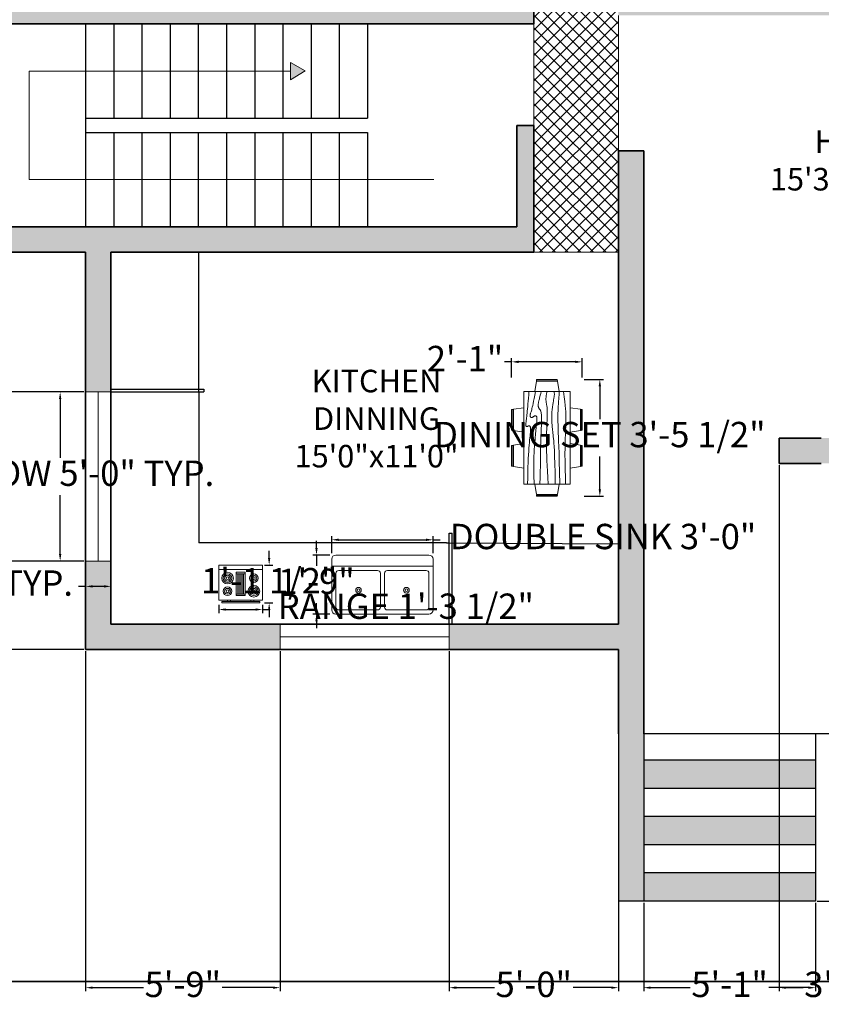
# Model space of a CAD drawing. Units: inches. Extents: x 1329 to 1989, y 1493 to 2072.
# Tile 2 of 4: x 1476 to 1761, y 1493 to 1842. Entities that reach past the tile are written whole.
import ezdxf

# ---------------------------------------------------------------- set-up
doc = ezdxf.new("R2010")
doc.units = ezdxf.units.IN
for name, color, linetype, lineweight in [('A-ANNO-DIMS', 2, 'Continuous', 18), ('A-ANNO-SYMB', 7, 'Continuous', 18), ('A-ANNO-TTLB', 7, 'Continuous', 35), ('A-AREA-IDEN', 7, 'Continuous', 25), ('A-EQPM', 8, 'Continuous', 18), ('A-FLOR', 7, 'Continuous', 25), ('A-FLOR-CASE', 8, 'Continuous', 25), ('A-FLOR-FIXT', 8, 'Continuous', 18), ('A-FLOR-STRS', 7, 'Continuous', 25), ('A-FURN', 8, 'Continuous', 18), ('A-GLAZ', 4, 'Continuous', 18), ('A-WALL', 7, 'Continuous', 35)]:
    doc.layers.add(name, color=color, linetype=linetype, lineweight=lineweight)
for name, color, linetype, lineweight, true_color in [('A-FLOR-PATT', 251, 'Continuous', 13, 0x636466), ('A-FLOR-STRS-PATT', 18, 'Continuous', 13, 0x000000), ('A-WALL-PATT', 251, 'Continuous', 13, 0x636466)]:
    doc.layers.add(name, color=color, linetype=linetype, lineweight=lineweight, true_color=true_color)
doc.styles.get("Standard").update_dxf_attribs({"font": 'arial.ttf'})
doc.dimstyles.new('ISO-25', dxfattribs={"dimtxt": 9, "dimasz": 2.5, "dimexe": 1.25, "dimexo": 0.625, "dimgap": 2, "dimtad": 0, "dimtih": 1, "dimtoh": 1, "dimdec": 1, "dimlunit": 4, "dimtxsty": 'Standard', "dimcen": 2.5, "dimadec": 0, "dimazin": 0, "dimtfac": 0.5, "dimtdec": 1, "dimtmove": 0, "dimatfit": 3, "dimfxl": 1, "dimarcsym": 0})

# ---------------------------------------------------------------- blocks, each defined once
blk = doc.blocks.new('Dining Set - 36 x 72 in.')
for p, q in [((-22.2343, 26.00059), (-23.4847, 17.99762)), ((-22.2304, 26), (-5.7608, 26)), ((-22, 27.5), (-22.1562, 26.50042)), ((-5.8416, 26.5), (-22.1534, 26.5)), ((-22, 27.5), (-6, 27.5)), ((-5.8437, 26.49966), (-6, 27.5)), ((-4.5152, 17.99762), (-5.7655, 25.99926)), ((5.7657, 26.00059), (4.5153, 17.99762)), ((5.7696, 26), (22.2392, 26)), ((6, 27.5), (5.8438, 26.50042)), ((22.1584, 26.5), (5.8466, 26.5)), ((6, 27.5), (22, 27.5)), ((22.1563, 26.49966), (22, 27.5)), ((23.4848, 17.99762), (22.2345, 25.99926)), ((36, 18), (-36, 18)), ((-36, 18), (-36, -18)), ((36, -18), (36, 18)), ((-45.5, 8), (-44.5004, 8.15617)), ((-45.5, 8), (-45.5, -8)), ((-44.5, -8.15843), (-44.5, 8.15338)), ((-44.0006, 8.23428), (-35.9976, 9.48474)), ((-44, 8.23041), (-44, -8.23915)), ((44.0006, 8.23428), (35.9976, 9.48474)), ((44, 8.23041), (44, -8.23915)), ((44.5, -8.15843), (44.5, 8.15338)), ((45.5, 8), (44.5005, 8.15617)), ((45.5, 8), (45.5, -8)), ((-44.4997, -8.15631), (-45.5, -8)), ((-35.9976, -9.48476), (-43.9993, -8.2345)), ((35.9976, -9.48476), (43.9993, -8.2345)), ((44.4997, -8.15631), (45.5, -8)), ((-36, -18), (36, -18)), ((-22.2343, -26.0006), (-23.4847, -17.99762)), ((-4.5152, -17.99762), (-5.7655, -25.99928)), ((5.7657, -26.0006), (4.5153, -17.99762)), ((23.4848, -17.99762), (22.2345, -25.99928)), ((-22.2304, -26), (-5.7608, -26)), ((-22, -27.5), (-22.1562, -26.50044)), ((-5.8416, -26.5), (-22.1534, -26.5)), ((-22, -27.5), (-6, -27.5)), ((-5.8437, -26.49967), (-6, -27.5)), ((5.7696, -26), (22.2392, -26)), ((6, -27.5), (5.8438, -26.50044)), ((22.1584, -26.5), (5.8466, -26.5)), ((6, -27.5), (22, -27.5)), ((22.1563, -26.49967), (22, -27.5))]:
    blk.add_line(p, q)
for points in [[(-36, 15), (-31.1772, 14.97754), (-26.8079, 14.91406), (-22.8538, 14.81543), (-19.276, 14.6875), (-16.0362, 14.53613), (-13.0957, 14.36718), (-10.4159, 14.18652), (-7.9583, 14), (-5.6904, 13.81315), (-3.6035, 13.63021), (-1.6954, 13.45508), (0.0365, 13.29166), (1.5945, 13.14388), (2.9811, 13.01562), (4.1988, 12.9108), (5.25, 12.83333), (6.1393, 12.78613), (6.8802, 12.76823), (7.4883, 12.77767), (7.9792, 12.8125), (8.3685, 12.87077), (8.6719, 12.95052), (8.9049, 13.0498), (9.0833, 13.16666), (9.2205, 13.29899), (9.3216, 13.44401), (9.3895, 13.59879), (9.4271, 13.76041), (9.4373, 13.92594), (9.4232, 14.09245), (9.3875, 14.257), (9.3333, 14.41666), (9.2638, 14.56917), (9.1836, 14.71484), (9.0975, 14.85465), (9.0104, 14.98958), (8.9272, 15.1206), (8.8529, 15.2487), (8.7922, 15.37483), (8.75, 15.5), (8.7305, 15.62467), (8.7344, 15.74739), (8.7617, 15.86621), (8.8125, 15.97916), (8.8867, 16.08431), (8.9844, 16.17968), (9.1055, 16.26334), (9.25, 16.33333), (9.4189, 16.38802), (9.6172, 16.42708), (9.8506, 16.45052), (10.125, 16.45833), (10.4463, 16.45052), (10.8203, 16.42708), (11.2529, 16.38802), (11.75, 16.33333), (12.3184, 16.26318), (12.9694, 16.17838), (13.7151, 16.07991), (14.5677, 15.96875), (15.5395, 15.84586), (16.6426, 15.71224), (17.8893, 15.56884), (19.2917, 15.41666), (20.859, 15.25667), (22.5879, 15.08984), (24.4721, 14.91715), (26.5052, 14.73958), (28.6809, 14.5581), (30.9929, 14.3737), (33.4347, 14.18733), (36, 14)], [(-36, 10), (-28.9766, 10.14274), (-23.1725, 10.20442), (-18.4241, 10.19775), (-14.5677, 10.13541), (-11.4399, 10.03011), (-8.877, 9.89453), (-6.7154, 9.74137), (-4.7917, 9.58333), (-2.9698, 9.43082), (-1.2246, 9.28515), (0.4415, 9.14534), (2.026, 9.01041), (3.5266, 8.87939), (4.9408, 8.7513), (6.266, 8.62516), (7.5, 8.5), (8.6411, 8.37549), (9.6914, 8.2539), (10.6538, 8.13818), (11.5312, 8.03125), (12.3267, 7.93603), (13.043, 7.85547), (13.6831, 7.79248), (14.25, 7.75), (14.7471, 7.7303), (15.1797, 7.73307), (15.5537, 7.75732), (15.875, 7.80208), (16.1494, 7.86637), (16.3828, 7.94922), (16.5811, 8.04964), (16.75, 8.16666), (16.8944, 8.29915), (17.0143, 8.44531), (17.1089, 8.60319), (17.1771, 8.77083), (17.218, 8.94629), (17.2305, 9.1276), (17.2137, 9.31282), (17.1667, 9.5), (17.0895, 9.6875), (16.987, 9.875), (16.8649, 10.0625), (16.7292, 10.25), (16.5856, 10.4375), (16.4401, 10.625), (16.2985, 10.8125), (16.1667, 11), (16.05, 11.18733), (15.9518, 11.3737), (15.8752, 11.5581), (15.8229, 11.73958), (15.798, 11.91715), (15.8034, 12.08984), (15.842, 12.25667), (15.9167, 12.41666), (16.0295, 12.56836), (16.1784, 12.70833), (16.3605, 12.83268), (16.5729, 12.9375), (16.8127, 13.01888), (17.0768, 13.07291), (17.3625, 13.0957), (17.6667, 13.08333), (17.9894, 13.03312), (18.3418, 12.94726), (18.7382, 12.82918), (19.1927, 12.68229), (19.7195, 12.51001), (20.3327, 12.31575), (21.0465, 12.10294), (21.875, 11.875), (22.8357, 11.63354), (23.959, 11.37304), (25.2786, 11.08618), (26.8282, 10.76562), (28.6414, 10.40405), (30.752, 9.99414), (33.1936, 9.52856), (36, 9)], [(-36, 5.5), (-30.7157, 5.3348), (-26.069, 5.20963), (-21.9946, 5.11767), (-18.4271, 5.05208), (-15.3009, 5.00602), (-12.5508, 4.97265), (-10.1112, 4.94515), (-7.9167, 4.91666), (-5.909, 4.88167), (-4.0586, 4.83984), (-2.3429, 4.79215), (-0.7396, 4.73958), (0.7739, 4.6831), (2.22, 4.6237), (3.6213, 4.56233), (5, 4.5), (6.373, 4.43782), (7.7344, 4.3776), (9.0723, 4.32129), (10.375, 4.27083), (11.6309, 4.22819), (12.8281, 4.19531), (13.9551, 4.17415), (15, 4.16666), (15.954, 4.17448), (16.819, 4.19791), (17.6001, 4.23698), (18.3021, 4.29166), (18.9299, 4.36198), (19.4883, 4.44791), (19.9823, 4.54948), (20.4167, 4.66666), (20.7969, 4.79899), (21.1302, 4.94401), (21.4245, 5.09879), (21.6875, 5.26041), (21.9271, 5.42594), (22.1511, 5.59245), (22.3672, 5.757), (22.5834, 5.91666), (22.8065, 6.06868), (23.0404, 6.21093), (23.2879, 6.34147), (23.5521, 6.45833), (23.8358, 6.55957), (24.142, 6.64323), (24.4735, 6.70735), (24.8334, 6.75), (25.2235, 6.76969), (25.642, 6.76692), (26.0858, 6.74267), (26.5521, 6.69791), (27.0379, 6.63362), (27.5404, 6.55078), (28.0565, 6.45036), (28.5834, 6.33333), (29.1242, 6.19987), (29.7071, 6.04687), (30.3661, 5.87044), (31.1354, 5.66666), (32.0493, 5.43164), (33.142, 5.16146), (34.4475, 4.85221), (36, 4.5)], [(-36, -1), (-30.7915, -0.6591), (-26.0195, -0.38216), (-21.6519, -0.16284), (-17.6563, 0.00521), (-14.0005, 0.12833), (-10.6523, 0.21289), (-7.5796, 0.26522), (-4.75, 0.29166), (-2.134, 0.29793), (0.2878, 0.28711), (2.5317, 0.26163), (4.6146, 0.22396), (6.5529, 0.17651), (8.3633, 0.12174), (10.0623, 0.06209), (11.6667, 0), (13.1899, -0.06201), (14.6341, -0.1211), (15.9982, -0.17432), (17.2813, -0.21875), (18.4823, -0.25147), (19.6003, -0.26953), (20.6343, -0.27002), (21.5834, -0.25), (22.4481, -0.20768), (23.2357, -0.14584), (23.9549, -0.06836), (24.6146, 0.02083), (25.2235, 0.11784), (25.7904, 0.21875), (26.3241, 0.31966), (26.8334, 0.41666), (27.3265, 0.50618), (27.8099, 0.58593), (28.2894, 0.65397), (28.7709, 0.70833), (29.2601, 0.74707), (29.763, 0.76823), (30.2855, 0.76985), (30.8334, 0.75), (31.4088, 0.70784), (31.9994, 0.64713), (32.589, 0.57275), (33.1615, 0.48958), (33.7008, 0.4025), (34.1908, 0.3164), (34.6153, 0.23616), (34.9584, 0.16666), (35.2099, 0.11165), (35.3848, 0.07031), (35.504, 0.04069), (35.5886, 0.02083), (35.6594, 0.00879), (35.7377, 0.0026), (35.8442, 0.00032), (36, 0)], [(-36, -6.5), (-27.1843, -6.31267), (-20.084, -6.1263), (-14.469, -5.9419), (-10.1094, -5.76042), (-6.7752, -5.58285), (-4.2363, -5.41016), (-2.2629, -5.24333), (-0.625, -5.08334), (0.8708, -4.93099), (2.2715, -4.78646), (3.5872, -4.64974), (4.8281, -4.52084), (6.0046, -4.39974), (7.127, -4.28646), (8.2053, -4.18099), (9.25, -4.08334), (10.2705, -3.99382), (11.2734, -3.91407), (12.2647, -3.84603), (13.25, -3.79167), (14.2354, -3.75293), (15.2266, -3.73177), (16.2295, -3.73015), (17.25, -3.75), (18.2912, -3.79248), (19.3451, -3.85547), (20.4009, -3.93604), (21.4479, -4.03125), (22.4754, -4.13819), (23.4727, -4.25391), (24.4289, -4.37549), (25.3334, -4.5), (26.1785, -4.62492), (26.9694, -4.74935), (27.7145, -4.87281), (28.4219, -4.99479), (29.1, -5.11483), (29.7572, -5.23242), (30.4016, -5.34709), (31.0417, -5.45834), (31.6837, -5.56437), (32.3262, -5.65821), (32.9658, -5.73153), (33.599, -5.77604), (34.2224, -5.78345), (34.8327, -5.74545), (35.4264, -5.65373), (36, -5.5)], [(-36, -10), (-26.4022, -9.81299), (-18.4675, -9.62891), (-11.9839, -9.45069), (-6.7396, -9.28125), (-2.5226, -9.12354), (0.8789, -8.98047), (3.6769, -8.85498), (6.0833, -8.75), (8.2767, -8.66765), (10.3021, -8.60677), (12.1712, -8.56543), (13.8958, -8.54167), (15.4876, -8.53353), (16.9583, -8.53907), (18.3197, -8.55632), (19.5834, -8.58334), (20.7616, -8.61841), (21.8685, -8.66081), (22.9188, -8.71004), (23.9271, -8.76563), (24.9081, -8.82707), (25.8763, -8.89388), (26.8465, -8.96558), (27.8334, -9.04167), (28.8474, -9.12118), (29.8828, -9.20117), (30.93, -9.27824), (31.9792, -9.34896), (33.0205, -9.40991), (34.0443, -9.45768), (35.0407, -9.48885), (36, -9.5)], [(-36, -14.5), (-30.0881, -14.33513), (-25.0332, -14.21224), (-20.7312, -14.12647), (-17.0781, -14.07292), (-13.97, -14.04671), (-11.3027, -14.04297), (-8.9724, -14.05681), (-6.875, -14.08334), (-4.9224, -14.11833), (-3.0905, -14.16016), (-1.3709, -14.20785), (0.2448, -14.26042), (1.7647, -14.3169), (3.1973, -14.3763), (4.5507, -14.43767), (5.8333, -14.5), (7.0554, -14.5621), (8.235, -14.62175), (9.3922, -14.67652), (10.5469, -14.72396), (11.7192, -14.76164), (12.929, -14.78711), (14.1965, -14.79794), (15.5417, -14.79167), (16.9933, -14.76424), (18.6152, -14.70508), (20.4804, -14.60197), (22.6615, -14.44271), (25.2312, -14.21509), (28.2624, -13.9069), (31.8277, -13.50594), (36, -13)]]:
    blk.add_lwpolyline(points)
blk = doc.blocks.new('Range-Oven - 30 in top')
for p, q in [((0, -3), (30, -3)), ((12, -6), (18, -6)), ((13, -20), (13, -6)), ((14, -6), (14, -20)), ((15, -20), (15, -6)), ((16, -6), (16, -20)), ((17, -20), (17, -6)), ((18, -20), (12, -20)), ((6, -24), (6, -25)), ((8, -25), (8, -24)), ((22, -25), (22, -24)), ((24, -24), (24, -25))]:
    blk.add_line(p, q)
for points in [[(0, -24), (0, 0), (30, 0), (30, -24)], [(12, -21), (12, -5), (18, -5), (18, -21)], [(2, -26), (2, -25), (28, -25), (28, -26)]]:
    blk.add_lwpolyline(points, close=True)
for centre, radius in [((6, -9), 4), ((6, -9), 3), ((24, -9), 3), ((6, -9), 2), ((6, -9), 1), ((24, -9), 2), ((24, -9), 1), ((6, -18), 3), ((6, -18), 2), ((6, -18), 1), ((24, -18), 4), ((24, -18), 3), ((24, -18), 2), ((24, -18), 1)]:
    blk.add_circle(centre, radius)
blk = doc.blocks.new('Sink-double - 36 in top')
for p, q in [((-18, -4), (18, -4)), ((-0.75, -18.5), (-0.75, -6.5)), ((0.75, -6.5), (0.75, -18.5))]:
    blk.add_line(p, q)
for points in [[(-16.5, 0), (16.5, 0)], [(-18, -19.5), (-18, -1.5)], [(18, -1.5), (18, -19.5)], [(-16.5, -18.5), (-16.5, -6.5)], [(-15.5, -5.5), (-1.75, -5.5)], [(1.75, -5.5), (15.5, -5.5)], [(16.5, -6.5), (16.5, -18.5)], [(-1.75, -19.5), (-15.5, -19.5)], [(15.5, -19.5), (1.75, -19.5)], [(16.5, -21), (-16.5, -21)]]:
    blk.add_lwpolyline(points)
for centre, radius in [((-8.5, -12.5), 1), ((-8.5, -12.5), 0.5), ((8.5, -12.5), 1), ((8.5, -12.5), 0.5)]:
    blk.add_circle(centre, radius)
for centre, radius, start, end in [((-16.5, -1.5), 1.5, 90, 180), ((16.5, -1.5), 1.5, 0, 90), ((-15.5, -6.5), 1, 90, 180), ((-1.75, -6.5), 1, 0, 90), ((1.75, -6.5), 1, 90, 180), ((15.5, -6.5), 1, 0, 90), ((-16.5, -19.5), 1.5, 180, 270), ((-15.5, -18.5), 1, 180, 270), ((-1.75, -18.5), 1, 270, 0), ((1.75, -18.5), 1, 180, 270), ((15.5, -18.5), 1, 270, 0), ((16.5, -19.5), 1.5, 270, 0)]:
    blk.add_arc(centre, radius, start, end)
blk = doc.blocks.new('*D14')
at = {"layer": 'A-ANNO-DIMS', "color": 0, "lineweight": -2, "transparency": 16777216}
for p, q in [((1499.06, 2002.52), (1370.79, 2002.52)), ((1372.04, 2000.02), (1372.04, 1817.12)), ((1372.04, 1621.02), (1372.04, 1803.93)), ((1499.06, 1618.52), (1370.79, 1618.52))]:
    blk.add_line(p, q, dxfattribs=at)
at = {"layer": 'A-ANNO-DIMS', "color": 0, "transparency": 16777216}
for points in [[(1371.62, 2000.02), (1372.45, 2000.02), (1372.04, 2002.52)], [(1371.62, 1621.02), (1372.45, 1621.02), (1372.04, 1618.52)]]:
    blk.add_solid(points, dxfattribs=at)
at = {"layer": 'Defpoints', "color": 0, "transparency": 16777216}
for p in [(1499.69, 2002.52), (1372.04, 1618.52), (1499.69, 1618.52)]:
    blk.add_point(p, dxfattribs=at)
at = {"layer": 'A-ANNO-DIMS', "color": 0, "transparency": 16777216, "insert": (1372.04, 1810.52), "char_height": 9, "attachment_point": 5}
blk.add_mtext("32'", dxfattribs=at)
blk = doc.blocks.new('WIN-60IN')
for p, q in [((0, 0), (0, 9)), ((60, 0), (60, 9)), ((0, 4.5), (60, 4.5))]:
    blk.add_line(p, q)
blk = doc.blocks.new('*D17')
at = {"layer": 'A-ANNO-DIMS', "color": 0, "lineweight": -2, "transparency": 16777216}
for p, q in [((1499.06, 1709.88), (1489.44, 1709.88)), ((1490.69, 1707.38), (1490.69, 1686.53)), ((1490.69, 1652.38), (1490.69, 1673.22)), ((1499.06, 1649.88), (1489.44, 1649.88))]:
    blk.add_line(p, q, dxfattribs=at)
at = {"layer": 'A-ANNO-DIMS', "color": 0, "transparency": 16777216}
for points in [[(1490.27, 1707.38), (1491.1, 1707.38), (1490.69, 1709.88)], [(1490.27, 1652.38), (1491.1, 1652.38), (1490.69, 1649.88)]]:
    blk.add_solid(points, dxfattribs=at)
at = {"layer": 'Defpoints', "color": 0, "transparency": 16777216}
for p in [(1490.69, 1709.88), (1499.69, 1709.88), (1499.69, 1649.88)]:
    blk.add_point(p, dxfattribs=at)
at = {"layer": 'A-ANNO-DIMS', "color": 0, "transparency": 16777216, "insert": (1490.69, 1679.88), "char_height": 9, "attachment_point": 5}
blk.add_mtext('WINDOW 5\'-0" TYP.', dxfattribs=at)
blk = doc.blocks.new('*D18')
at = {"layer": 'A-ANNO-DIMS', "color": 0, "lineweight": -2, "transparency": 16777216}
for p, q in [((1499.69, 1649.25), (1499.69, 1639.63)), ((1508.69, 1649.25), (1508.69, 1639.63)), ((1499.69, 1640.88), (1497.19, 1640.88)), ((1506.19, 1640.88), (1502.19, 1640.88))]:
    blk.add_line(p, q, dxfattribs=at)
at = {"layer": 'A-ANNO-DIMS', "color": 0, "transparency": 16777216}
for points in [[(1502.19, 1641.29), (1502.19, 1640.46), (1499.69, 1640.88)], [(1506.19, 1641.29), (1506.19, 1640.46), (1508.69, 1640.88)]]:
    blk.add_solid(points, dxfattribs=at)
at = {"layer": 'Defpoints', "color": 0, "transparency": 16777216}
for p in [(1499.69, 1649.88), (1508.69, 1649.88), (1499.69, 1640.88)]:
    blk.add_point(p, dxfattribs=at)
at = {"layer": 'A-ANNO-DIMS', "color": 0, "transparency": 16777216, "insert": (1467.76, 1640.88), "char_height": 9, "attachment_point": 5}
blk.add_mtext('0\'-9" TYP.', dxfattribs=at)
blk = doc.blocks.new('*D27')
at = {"layer": 'A-ANNO-DIMS', "color": 0, "lineweight": -2, "transparency": 16777216}
for p, q in [((1676.53, 1714.35), (1683.38, 1714.35)), ((1682.13, 1711.85), (1682.13, 1700.26)), ((1682.13, 1675.36), (1682.13, 1686.95)), ((1676.53, 1672.86), (1683.38, 1672.86))]:
    blk.add_line(p, q, dxfattribs=at)
at = {"layer": 'A-ANNO-DIMS', "color": 0, "transparency": 16777216}
for points in [[(1681.71, 1711.85), (1682.55, 1711.85), (1682.13, 1714.35)], [(1681.71, 1675.36), (1682.55, 1675.36), (1682.13, 1672.86)]]:
    blk.add_solid(points, dxfattribs=at)
at = {"layer": 'Defpoints', "color": 0, "transparency": 16777216}
for p in [(1675.9, 1714.35), (1682.13, 1714.35), (1675.9, 1672.86)]:
    blk.add_point(p, dxfattribs=at)
at = {"layer": 'A-ANNO-DIMS', "color": 0, "transparency": 16777216, "insert": (1682.13, 1693.6), "char_height": 9, "attachment_point": 5}
blk.add_mtext('DINING SET 3\'-5 1/2"', dxfattribs=at)
blk = doc.blocks.new('*D28')
at = {"layer": 'A-ANNO-DIMS', "color": 0, "lineweight": -2, "transparency": 16777216}
for p, q in [((1650.82, 1720.58), (1648.32, 1720.58)), ((1650.82, 1714.98), (1650.82, 1721.83)), ((1673.4, 1720.58), (1653.32, 1720.58)), ((1675.9, 1714.98), (1675.9, 1721.83))]:
    blk.add_line(p, q, dxfattribs=at)
at = {"layer": 'A-ANNO-DIMS', "color": 0, "transparency": 16777216}
for points in [[(1653.32, 1720.99), (1653.32, 1720.16), (1650.82, 1720.58)], [(1673.4, 1720.99), (1673.4, 1720.16), (1675.9, 1720.58)]]:
    blk.add_solid(points, dxfattribs=at)
at = {"layer": 'Defpoints', "color": 0, "transparency": 16777216}
for p in [(1650.82, 1720.58), (1650.82, 1714.35), (1675.9, 1714.35)]:
    blk.add_point(p, dxfattribs=at)
at = {"layer": 'A-ANNO-DIMS', "color": 0, "transparency": 16777216, "insert": (1634.29, 1720.58), "char_height": 9, "attachment_point": 5}
blk.add_mtext('2\'-1"', dxfattribs=at)
blk = doc.blocks.new('*D31')
at = {"layer": 'A-ANNO-DIMS', "color": 0, "lineweight": -2, "transparency": 16777216}
for p, q in [((1546.95, 1634.37), (1546.95, 1631.42)), ((1549.45, 1632.67), (1559.99, 1632.67)), ((1562.49, 1634.37), (1562.49, 1631.42)), ((1562.49, 1632.67), (1564.99, 1632.67))]:
    blk.add_line(p, q, dxfattribs=at)
at = {"layer": 'A-ANNO-DIMS', "color": 0, "transparency": 16777216}
for points in [[(1549.45, 1633.08), (1549.45, 1632.25), (1546.95, 1632.67)], [(1559.99, 1633.08), (1559.99, 1632.25), (1562.49, 1632.67)]]:
    blk.add_solid(points, dxfattribs=at)
at = {"layer": 'Defpoints', "color": 0, "transparency": 16777216}
for p in [(1546.95, 1635), (1562.49, 1635), (1562.49, 1632.67)]:
    blk.add_point(p, dxfattribs=at)
at = {"layer": 'A-ANNO-DIMS', "color": 0, "transparency": 16777216, "insert": (1613.31, 1632.67), "char_height": 9, "attachment_point": 5}
blk.add_mtext('RANGE 1\'-3 1/2"', dxfattribs=at)
blk = doc.blocks.new('*D32')
at = {"layer": 'A-ANNO-DIMS', "color": 0, "lineweight": -2, "transparency": 16777216}
for p, q in [((1564.83, 1650.97), (1564.83, 1653.47)), ((1563.12, 1648.47), (1566.08, 1648.47)), ((1564.83, 1648.47), (1564.83, 1648.39)), ((1563.12, 1635), (1566.08, 1635)), ((1564.83, 1635), (1564.83, 1635.08)), ((1564.83, 1632.5), (1564.83, 1630))]:
    blk.add_line(p, q, dxfattribs=at)
at = {"layer": 'A-ANNO-DIMS', "color": 0, "transparency": 16777216}
for points in [[(1564.41, 1650.97), (1565.24, 1650.97), (1564.83, 1648.47)], [(1564.41, 1632.5), (1565.24, 1632.5), (1564.83, 1635)]]:
    blk.add_solid(points, dxfattribs=at)
at = {"layer": 'Defpoints', "color": 0, "transparency": 16777216}
for p in [(1562.49, 1648.47), (1564.83, 1648.47), (1562.49, 1635)]:
    blk.add_point(p, dxfattribs=at)
at = {"layer": 'A-ANNO-DIMS', "color": 0, "transparency": 16777216, "insert": (1564.83, 1641.73), "char_height": 9, "attachment_point": 5}
blk.add_mtext('1\'-1 1/2"', dxfattribs=at)
blk = doc.blocks.new('*D33')
at = {"layer": 'A-ANNO-DIMS', "color": 0, "lineweight": -2, "transparency": 16777216}
for p, q in [((1587.01, 1652.65), (1587.01, 1658.67)), ((1589.51, 1657.42), (1620.51, 1657.42)), ((1623.01, 1652.65), (1623.01, 1658.67)), ((1623.01, 1657.42), (1625.51, 1657.42))]:
    blk.add_line(p, q, dxfattribs=at)
at = {"layer": 'A-ANNO-DIMS', "color": 0, "transparency": 16777216}
for points in [[(1589.51, 1657.84), (1589.51, 1657), (1587.01, 1657.42)], [(1620.51, 1657.84), (1620.51, 1657), (1623.01, 1657.42)]]:
    blk.add_solid(points, dxfattribs=at)
at = {"layer": 'Defpoints', "color": 0, "transparency": 16777216}
for p in [(1623.01, 1657.42), (1587.01, 1652.02), (1623.01, 1652.02)]:
    blk.add_point(p, dxfattribs=at)
at = {"layer": 'A-ANNO-DIMS', "color": 0, "transparency": 16777216, "insert": (1683.27, 1657.42), "char_height": 9, "attachment_point": 5}
blk.add_mtext('DOUBLE SINK 3\'-0"', dxfattribs=at)
blk = doc.blocks.new('*D34')
at = {"layer": 'A-ANNO-DIMS', "color": 0, "lineweight": -2, "transparency": 16777216}
for p, q in [((1581.61, 1654.52), (1581.61, 1657.02)), ((1586.39, 1652.02), (1580.36, 1652.02)), ((1581.61, 1652.02), (1581.61, 1648.12)), ((1581.61, 1631.02), (1581.61, 1634.93)), ((1586.39, 1631.02), (1580.36, 1631.02)), ((1581.61, 1628.52), (1581.61, 1626.02))]:
    blk.add_line(p, q, dxfattribs=at)
at = {"layer": 'A-ANNO-DIMS', "color": 0, "transparency": 16777216}
for points in [[(1581.2, 1654.52), (1582.03, 1654.52), (1581.61, 1652.02)], [(1581.2, 1628.52), (1582.03, 1628.52), (1581.61, 1631.02)]]:
    blk.add_solid(points, dxfattribs=at)
at = {"layer": 'Defpoints', "color": 0, "transparency": 16777216}
for p in [(1581.61, 1652.02), (1587.01, 1652.02), (1587.01, 1631.02)]:
    blk.add_point(p, dxfattribs=at)
at = {"layer": 'A-ANNO-DIMS', "color": 0, "transparency": 16777216, "insert": (1581.61, 1641.52), "char_height": 9, "attachment_point": 5}
blk.add_mtext('1\'-9"', dxfattribs=at)
blk = doc.blocks.new('*D38')
at = {"layer": 'A-ANNO-DIMS', "color": 0, "lineweight": -2, "transparency": 16777216}
for p, q in [((1890.31, 2002.52), (1921.64, 2002.52)), ((1920.39, 2000.02), (1920.39, 1772.49)), ((1920.39, 1531.65), (1920.39, 1759.18)), ((1759.27, 1529.15), (1921.64, 1529.15))]:
    blk.add_line(p, q, dxfattribs=at)
at = {"layer": 'A-ANNO-DIMS', "color": 0, "transparency": 16777216}
for points in [[(1919.97, 2000.02), (1920.8, 2000.02), (1920.39, 2002.52)], [(1919.97, 1531.65), (1920.8, 1531.65), (1920.39, 1529.15)]]:
    blk.add_solid(points, dxfattribs=at)
at = {"layer": 'Defpoints', "color": 0, "transparency": 16777216}
for p in [(1889.69, 2002.52), (1758.64, 1529.15), (1920.39, 1529.15)]:
    blk.add_point(p, dxfattribs=at)
at = {"layer": 'A-ANNO-DIMS', "color": 0, "transparency": 16777216, "insert": (1920.39, 1765.84), "char_height": 9, "attachment_point": 5}
blk.add_mtext('39\'-5 1/2"', dxfattribs=at)
blk = doc.blocks.new('*D49')
at = {"layer": 'A-ANNO-DIMS', "color": 0, "lineweight": -2, "transparency": 16777216}
for p, q in [((1499.06, 1759.52), (1374.19, 1759.52)), ((1375.44, 1757.02), (1375.44, 1741.35)), ((1375.44, 1712.38), (1375.44, 1728.05)), ((1499.06, 1709.88), (1374.19, 1709.88))]:
    blk.add_line(p, q, dxfattribs=at)
at = {"layer": 'A-ANNO-DIMS', "color": 0, "transparency": 16777216}
for points in [[(1375.02, 1757.02), (1375.86, 1757.02), (1375.44, 1759.52)], [(1375.02, 1712.38), (1375.86, 1712.38), (1375.44, 1709.88)]]:
    blk.add_solid(points, dxfattribs=at)
at = {"layer": 'Defpoints', "color": 0, "transparency": 16777216}
for p in [(1375.44, 1759.52), (1499.69, 1759.52), (1499.69, 1709.88)]:
    blk.add_point(p, dxfattribs=at)
at = {"layer": 'A-ANNO-DIMS', "color": 0, "transparency": 16777216, "insert": (1375.44, 1734.7), "char_height": 9, "attachment_point": 5}
blk.add_mtext('4\'-1 1/2"', dxfattribs=at)
blk = doc.blocks.new('*D50')
at = {"layer": 'A-ANNO-DIMS', "color": 0, "lineweight": -2, "transparency": 16777216}
for p, q in [((1499.06, 1649.88), (1374.19, 1649.88)), ((1375.44, 1647.38), (1375.44, 1640.85)), ((1375.44, 1621.02), (1375.44, 1627.55)), ((1499.06, 1618.52), (1374.19, 1618.52))]:
    blk.add_line(p, q, dxfattribs=at)
at = {"layer": 'A-ANNO-DIMS', "color": 0, "transparency": 16777216}
for points in [[(1375.02, 1647.38), (1375.86, 1647.38), (1375.44, 1649.88)], [(1375.02, 1621.02), (1375.86, 1621.02), (1375.44, 1618.52)]]:
    blk.add_solid(points, dxfattribs=at)
at = {"layer": 'Defpoints', "color": 0, "transparency": 16777216}
for p in [(1499.69, 1649.88), (1375.44, 1618.52), (1499.69, 1618.52)]:
    blk.add_point(p, dxfattribs=at)
at = {"layer": 'A-ANNO-DIMS', "color": 0, "transparency": 16777216, "insert": (1375.44, 1634.2), "char_height": 9, "attachment_point": 5}
blk.add_mtext('2\'-7 1/2"', dxfattribs=at)
blk = doc.blocks.new('*D51')
at = {"layer": 'A-ANNO-DIMS', "color": 0, "lineweight": -2, "transparency": 16777216}
for p, q in [((1499.69, 1617.9), (1499.69, 1497.2)), ((1568.69, 1617.9), (1568.69, 1497.2)), ((1502.19, 1498.45), (1520.22, 1498.45)), ((1566.19, 1498.45), (1548.15, 1498.45))]:
    blk.add_line(p, q, dxfattribs=at)
at = {"layer": 'A-ANNO-DIMS', "color": 0, "transparency": 16777216}
for points in [[(1502.19, 1498.87), (1502.19, 1498.03), (1499.69, 1498.45)], [(1566.19, 1498.87), (1566.19, 1498.03), (1568.69, 1498.45)]]:
    blk.add_solid(points, dxfattribs=at)
at = {"layer": 'Defpoints', "color": 0, "transparency": 16777216}
for p in [(1499.69, 1618.52), (1568.69, 1618.52), (1568.69, 1498.45)]:
    blk.add_point(p, dxfattribs=at)
at = {"layer": 'A-ANNO-DIMS', "color": 0, "transparency": 16777216, "insert": (1534.19, 1498.45), "char_height": 9, "attachment_point": 5}
blk.add_mtext('5\'-9"', dxfattribs=at)
blk = doc.blocks.new('*D52')
at = {"layer": 'A-ANNO-DIMS', "color": 0, "lineweight": -2, "transparency": 16777216}
for p, q in [((1628.69, 1617.9), (1628.69, 1497.2)), ((1688.69, 1617.9), (1688.69, 1497.2)), ((1631.19, 1498.45), (1644.72, 1498.45)), ((1686.19, 1498.45), (1672.65, 1498.45))]:
    blk.add_line(p, q, dxfattribs=at)
at = {"layer": 'A-ANNO-DIMS', "color": 0, "transparency": 16777216}
for points in [[(1631.19, 1498.87), (1631.19, 1498.03), (1628.69, 1498.45)], [(1686.19, 1498.87), (1686.19, 1498.03), (1688.69, 1498.45)]]:
    blk.add_solid(points, dxfattribs=at)
at = {"layer": 'Defpoints', "color": 0, "transparency": 16777216}
for p in [(1628.69, 1618.52), (1688.69, 1618.52), (1688.69, 1498.45)]:
    blk.add_point(p, dxfattribs=at)
at = {"layer": 'A-ANNO-DIMS', "color": 0, "transparency": 16777216, "insert": (1658.69, 1498.45), "char_height": 9, "attachment_point": 5}
blk.add_mtext('5\'-0"', dxfattribs=at)
blk = doc.blocks.new('*D53')
at = {"layer": 'A-ANNO-DIMS', "color": 0, "lineweight": -2, "transparency": 16777216}
for p, q in [((1697.69, 1528.52), (1697.69, 1497.2)), ((1758.64, 1528.52), (1758.64, 1497.2)), ((1700.19, 1498.45), (1714.2, 1498.45)), ((1756.14, 1498.45), (1742.13, 1498.45))]:
    blk.add_line(p, q, dxfattribs=at)
at = {"layer": 'A-ANNO-DIMS', "color": 0, "transparency": 16777216}
for points in [[(1700.19, 1498.87), (1700.19, 1498.03), (1697.69, 1498.45)], [(1756.14, 1498.87), (1756.14, 1498.03), (1758.64, 1498.45)]]:
    blk.add_solid(points, dxfattribs=at)
at = {"layer": 'Defpoints', "color": 0, "transparency": 16777216}
for p in [(1697.69, 1529.15), (1758.64, 1529.15), (1758.64, 1498.45)]:
    blk.add_point(p, dxfattribs=at)
at = {"layer": 'A-ANNO-DIMS', "color": 0, "transparency": 16777216, "insert": (1728.16, 1498.45), "char_height": 9, "attachment_point": 5}
blk.add_mtext('5\'-1"', dxfattribs=at)
blk = doc.blocks.new('*D54')
at = {"layer": 'A-ANNO-DIMS', "color": 0, "lineweight": -2, "transparency": 16777216}
for p, q in [((1745.69, 1683.9), (1745.69, 1497.2)), ((1790.69, 1683.9), (1790.69, 1497.2)), ((1748.19, 1498.45), (1754.23, 1498.45)), ((1788.19, 1498.45), (1782.15, 1498.45))]:
    blk.add_line(p, q, dxfattribs=at)
at = {"layer": 'A-ANNO-DIMS', "color": 0, "transparency": 16777216}
for points in [[(1748.19, 1498.87), (1748.19, 1498.03), (1745.69, 1498.45)], [(1788.19, 1498.87), (1788.19, 1498.03), (1790.69, 1498.45)]]:
    blk.add_solid(points, dxfattribs=at)
at = {"layer": 'Defpoints', "color": 0, "transparency": 16777216}
for p in [(1745.69, 1684.52), (1790.69, 1684.52), (1790.69, 1498.45)]:
    blk.add_point(p, dxfattribs=at)
at = {"layer": 'A-ANNO-DIMS', "color": 0, "transparency": 16777216, "insert": (1768.19, 1498.45), "char_height": 9, "attachment_point": 5}
blk.add_mtext('3\'-9"', dxfattribs=at)

msp = doc.modelspace()

# ---------------------------------------------------------------- hatches: boundary and pattern name
at = {"layer": 'A-ANNO-SYMB'}
h = msp.add_hatch(color=256, dxfattribs=at)
h.dxf.hatch_style = 1
h.paths.add_polyline_path([(1572.39, 1826.82), (1572.39, 1823.77), (1572.39, 1820.71), (1577.59, 1823.83)])
at = {"layer": 'A-FLOR-PATT'}
h = msp.add_hatch(dxfattribs=at)
h.set_pattern_fill('ANSI37', color=256)
h.paths.add_polyline_path([(1754.69, 1885.52), (1754.69, 1939.52), (1730.69, 1939.52), (1712.69, 1939.52), (1712.69, 1909.52), (1712.69, 1903.52), (1706.69, 1903.52), (1658.69, 1903.52), (1658.69, 1885.52), (1658.69, 1804.52), (1658.69, 1759.52), (1688.69, 1759.52), (1688.69, 1795.52), (1688.69, 1843.52), (1688.69, 1849.52), (1754.69, 1849.52)])
h.paths.add_polyline_path([(1677.05, 1890.24), (1661.98, 1890.24, -0.414214), (1661.14, 1891.07), (1661.14, 1900.56, -0.414214), (1661.98, 1901.4), (1677.05, 1901.4, -0.414214), (1677.89, 1900.56), (1677.89, 1891.07, -0.414214)], flags=16)
h.paths.add_polyline_path([(1676.49, 1891.07), (1662.54, 1891.07, -0.414214), (1661.98, 1891.63), (1661.98, 1897.77, -0.414214), (1662.54, 1898.33), (1676.49, 1898.33, -0.414214), (1677.05, 1897.77), (1677.05, 1891.63, -0.414214)], flags=0)
h.paths.add_polyline_path([(1668.96, 1894.7, -1), (1670.07, 1894.7, -1)], flags=0)
h.paths.add_polyline_path([(1669.23, 1894.7, -1), (1669.79, 1894.7, -1)], flags=0)
at = {"layer": 'A-FLOR-STRS-PATT'}
h = msp.add_hatch(color=256, dxfattribs=at)
h.dxf.hatch_style = 1
h.paths.add_polyline_path([(1758.64, 1539.15), (1697.69, 1539.15), (1697.69, 1529.15), (1758.64, 1529.15)])
h.paths.add_polyline_path([(1758.64, 1559.15), (1697.69, 1559.15), (1697.69, 1549.15), (1758.64, 1549.15)])
h.paths.add_polyline_path([(1758.64, 1579.15), (1697.69, 1579.15), (1697.69, 1569.15), (1758.64, 1569.15)])
at = {"layer": 'A-WALL-PATT'}
h = msp.add_hatch(color=256, dxfattribs=at)
h.dxf.hatch_style = 1
h.paths.add_polyline_path([(1550.69, 2002.52), (1499.69, 2002.52), (1499.69, 1951.52), (1508.69, 1951.52), (1508.69, 1993.52), (1550.69, 1993.52)])
h.paths.add_polyline_path([(1670.69, 2002.52), (1610.69, 2002.52), (1610.69, 1993.52), (1652.69, 1993.52), (1652.69, 1885.52), (1658.69, 1885.52), (1658.69, 1903.52), (1706.69, 1903.52), (1712.69, 1903.52), (1712.69, 1909.52), (1706.69, 1909.52), (1658.69, 1909.52), (1658.69, 1993.52), (1670.69, 1993.52)])
h.paths.add_polyline_path([(1721.69, 2002.52), (1694.69, 2002.52), (1694.69, 1993.52), (1706.69, 1993.52), (1706.69, 1939.52), (1712.69, 1939.52), (1730.69, 1939.52), (1730.69, 1945.52), (1712.69, 1945.52), (1712.69, 1993.52), (1721.69, 1993.52)])
h.paths.add_polyline_path([(1790.69, 2002.52), (1745.69, 2002.52), (1745.69, 1993.52), (1754.69, 1993.52), (1754.69, 1945.52), (1754.69, 1939.52), (1754.69, 1885.52), (1760.69, 1885.52), (1760.69, 1993.52), (1790.69, 1993.52)])
h.paths.add_polyline_path([(1889.69, 2002.52), (1850.69, 2002.52), (1850.69, 1993.52), (1880.69, 1993.52), (1880.69, 1951.52), (1889.69, 1951.52)])
h.paths.add_polyline_path([(1889.69, 1891.52), (1880.69, 1891.52), (1880.69, 1849.52), (1760.69, 1849.52), (1754.69, 1849.52), (1688.69, 1849.52), (1688.69, 1843.52), (1697.69, 1843.52), (1760.69, 1843.52), (1880.69, 1843.52), (1880.69, 1798.52), (1889.69, 1798.52)])
h.paths.add_polyline_path([(1658.69, 1849.52), (1652.69, 1849.52), (1508.69, 1849.52), (1508.69, 1891.52), (1499.69, 1891.52), (1499.69, 1849.52), (1406.14, 1849.52), (1406.14, 1828.52), (1415.14, 1828.52), (1415.14, 1840.52), (1508.69, 1840.52), (1652.69, 1840.52), (1658.69, 1840.52)])
h.paths.add_polyline_path([(1658.69, 1804.52), (1652.69, 1804.52), (1652.69, 1768.52), (1508.69, 1768.52), (1415.14, 1768.52), (1415.14, 1780.52), (1406.14, 1780.52), (1406.14, 1759.52), (1499.69, 1759.52), (1499.69, 1709.88), (1508.69, 1709.88), (1508.69, 1759.52), (1658.69, 1759.52)])
h.paths.add_polyline_path([(1508.69, 1649.88), (1499.69, 1649.88), (1499.69, 1618.52), (1568.69, 1618.52), (1568.69, 1627.52), (1508.69, 1627.52)])
h.paths.add_polyline_path([(1697.69, 1684.52), (1697.69, 1693.52), (1697.69, 1795.52), (1688.69, 1795.52), (1688.69, 1693.52), (1688.69, 1684.52), (1688.69, 1627.52), (1628.69, 1627.52), (1628.69, 1618.52), (1688.69, 1618.52), (1688.69, 1588.52), (1697.69, 1588.52), (1697.69, 1618.52)])
h.paths.add_polyline_path([(1790.69, 1693.52), (1760.69, 1693.52), (1745.69, 1693.52), (1745.69, 1684.52), (1760.69, 1684.52), (1790.69, 1684.52)])
h.paths.add_polyline_path([(1889.69, 1738.52), (1880.69, 1738.52), (1880.69, 1693.52), (1850.69, 1693.52), (1850.69, 1684.52), (1880.69, 1684.52), (1889.69, 1684.52)])
h = msp.add_hatch(color=256, dxfattribs=at)
h.dxf.hatch_style = 1
h.paths.add_polyline_path([(1697.69, 1588.52), (1697.69, 1618.52), (1697.69, 1684.52), (1697.69, 1693.52), (1697.69, 1795.52), (1688.69, 1795.52), (1688.69, 1693.52), (1688.69, 1684.52), (1688.69, 1627.52), (1628.69, 1627.52), (1628.69, 1618.52), (1688.69, 1618.52), (1688.69, 1588.52), (1688.69, 1529.15), (1697.69, 1529.15)])

# ---------------------------------------------------------------- linework, layer by layer
at = {"layer": 'A-ANNO-SYMB'}
for p, q in [((1572.39, 1823.77), (1572.39, 1826.82)), ((1572.39, 1826.82), (1577.59, 1823.83)), ((1569.69, 1823.77), (1479.69, 1823.77)), ((1479.69, 1785.27), (1479.69, 1823.77)), ((1569.69, 1823.77), (1572.39, 1823.77)), ((1577.59, 1823.83), (1572.39, 1820.71)), ((1572.39, 1820.71), (1572.39, 1823.77)), ((1599.69, 1785.27), (1479.69, 1785.27)), ((1599.69, 1785.27), (1623.24, 1785.27))]:
    msp.add_line(p, q, dxfattribs=at)
at = {"layer": 'A-ANNO-TTLB'}
msp.add_lwpolyline([(1329.11, 2071.84), (1964.17, 2071.84), (1964.17, 1500.65), (1329.11, 1500.65)], close=True, dxfattribs=at)
at = {"layer": 'A-FLOR'}
msp.add_line((1889.69, 1588.52), (1697.69, 1588.52), dxfattribs=at)
at = {"layer": 'A-FLOR-CASE'}
for p, q in [((1539.93, 1709.88), (1539.93, 1759.52)), ((1508.69, 1710.88), (1541.61, 1710.88)), ((1508.69, 1709.88), (1541.61, 1709.88)), ((1539.93, 1709.88), (1539.93, 1656.33)), ((1541.61, 1710.88), (1541.61, 1709.88)), ((1628.69, 1627.52), (1628.69, 1659.78)), ((1628.69, 1659.78), (1629.69, 1659.78)), ((1629.69, 1627.52), (1629.69, 1659.78)), ((1627.69, 1656.33), (1539.93, 1656.33)), ((1627.69, 1656.33), (1628.69, 1656.33)), ((1628.69, 1656.33), (1688.69, 1656.02))]:
    msp.add_line(p, q, dxfattribs=at)
at = {"layer": 'A-FLOR-PATT'}
for p, q in [((1658.69, 1804.52), (1658.69, 1885.52)), ((1688.69, 1843.52), (1688.69, 1795.52)), ((1658.69, 1759.52), (1688.69, 1759.52))]:
    msp.add_line(p, q, dxfattribs=at)
at = {"layer": 'A-FLOR-STRS'}
for p, q in [((1499.69, 1840.52), (1499.69, 1768.52)), ((1509.69, 1840.52), (1509.69, 1807.02)), ((1519.69, 1840.52), (1519.69, 1807.02)), ((1529.69, 1840.52), (1529.69, 1807.02)), ((1539.69, 1840.52), (1539.69, 1807.02)), ((1549.69, 1840.52), (1549.69, 1807.02)), ((1559.69, 1840.52), (1559.69, 1807.02)), ((1569.69, 1840.52), (1569.69, 1807.02)), ((1579.69, 1840.52), (1579.69, 1807.02)), ((1589.69, 1840.52), (1589.69, 1807.02)), ((1599.69, 1840.52), (1599.69, 1807.02)), ((1499.69, 1807.02), (1599.69, 1807.02)), ((1499.69, 1802.02), (1599.69, 1802.02)), ((1509.69, 1802.02), (1509.69, 1768.52)), ((1519.69, 1802.02), (1519.69, 1768.52)), ((1529.69, 1802.02), (1529.69, 1768.52)), ((1539.69, 1802.02), (1539.69, 1768.52)), ((1549.69, 1802.02), (1549.69, 1768.52)), ((1559.69, 1802.02), (1559.69, 1768.52)), ((1569.69, 1802.02), (1569.69, 1768.52)), ((1579.69, 1802.02), (1579.69, 1768.52)), ((1589.69, 1802.02), (1589.69, 1768.52)), ((1599.69, 1802.02), (1599.69, 1768.52)), ((1688.69, 1588.52), (1688.69, 1529.15)), ((1697.69, 1588.52), (1697.69, 1529.15)), ((1758.64, 1588.52), (1758.64, 1529.15)), ((1758.64, 1579.15), (1697.69, 1579.15)), ((1758.64, 1569.15), (1697.69, 1569.15)), ((1758.64, 1559.15), (1697.69, 1559.15)), ((1758.64, 1549.15), (1697.69, 1549.15)), ((1758.64, 1539.15), (1697.69, 1539.15)), ((1758.64, 1529.15), (1688.69, 1529.15))]:
    msp.add_line(p, q, dxfattribs=at)
at = {"layer": 'A-WALL'}
for p, q in [((1658.69, 1849.52), (1658.69, 1840.52)), ((1508.69, 1840.52), (1415.14, 1840.52)), ((1508.69, 1840.52), (1652.69, 1840.52)), ((1652.69, 1840.52), (1658.69, 1840.52)), ((1652.69, 1804.52), (1652.69, 1768.52)), ((1652.69, 1804.52), (1658.69, 1804.52)), ((1658.69, 1804.52), (1658.69, 1759.52)), ((1688.69, 1795.52), (1688.69, 1768.52)), ((1697.69, 1795.52), (1688.69, 1795.52)), ((1688.69, 1795.52), (1688.69, 1693.52)), ((1697.69, 1795.52), (1697.69, 1693.52)), ((1508.69, 1768.52), (1415.14, 1768.52)), ((1508.69, 1768.52), (1652.69, 1768.52)), ((1499.69, 1759.52), (1406.14, 1759.52)), ((1499.69, 1759.52), (1499.69, 1618.52)), ((1508.69, 1759.52), (1658.69, 1759.52)), ((1508.69, 1759.52), (1508.69, 1627.52)), ((1688.69, 1693.52), (1688.69, 1684.52)), ((1697.69, 1693.52), (1697.69, 1684.52)), ((1760.69, 1693.52), (1745.69, 1693.52)), ((1745.69, 1693.52), (1745.69, 1684.52)), ((1688.69, 1684.52), (1688.69, 1627.52)), ((1697.69, 1684.52), (1697.69, 1618.52)), ((1760.69, 1684.52), (1745.69, 1684.52)), ((1508.69, 1627.52), (1688.69, 1627.52)), ((1499.69, 1618.52), (1688.69, 1618.52)), ((1688.69, 1618.52), (1688.69, 1588.52)), ((1697.69, 1618.52), (1697.69, 1588.52))]:
    msp.add_line(p, q, dxfattribs=at)

# ---------------------------------------------------------------- block references
at = {"layer": 'A-EQPM', "xscale": 0.5182011901776195, "yscale": 0.5182011901776195, "zscale": 0.5182011901776195}
msp.add_blockref('Range-Oven - 30 in top', (1546.95, 1648.47), dxfattribs=at)
at = {"layer": 'A-FLOR-FIXT'}
msp.add_blockref('Sink-double - 36 in top', (1605.01, 1652.02), dxfattribs=at)
at = {"layer": 'A-FURN', "xscale": 0.4560073290152355, "yscale": 0.4560073290152355, "zscale": 0.4560073290152355, "rotation": 90}
msp.add_blockref('Dining Set - 36 x 72 in.', (1663.36, 1693.6), dxfattribs=at)
at = {"layer": 'A-GLAZ'}
for p, rotation in [((1508.69, 1649.88), 90.00000000000011), ((1628.69, 1627.52), 180)]:
    msp.add_blockref('WIN-60IN', p, dxfattribs=dict(at, rotation=rotation))

# ---------------------------------------------------------------- texts
at = {"layer": 'A-AREA-IDEN', "char_height": 8, "attachment_point": 1}
for s, width, insert in [('\\pxqc;{\\fArial|b1|i0|c0|p34;HALL\\P15\'3"x12\'6"}', 85.2875, (1728.9, 1802.74)), ('\\pxqc;{\\fArial|b1|i0|c0|p34;KITCHEN\\PDINNING\\P15\'0"x11\'0"}', 81.4303, (1562.2, 1717.77))]:
    msp.add_mtext_dynamic_manual_height_columns(s, width=width, gutter_width=12.5, heights=[0], dxfattribs=dict(at, insert=insert))

# ---------------------------------------------------------------- dimensions: what is measured, and where the dimension line sits
at = {"layer": 'A-ANNO-DIMS'}
for base, p1, p2, angle, override, picture, middle in [((1372.04, 1618.52), (1499.69, 2002.52), (1499.69, 1618.52), 90, {"dimclrd": 0, "dimclre": 0, "dimclrt": 0}, '*D14', (1372.04, 1810.52)), ((1920.39, 1529.15), (1889.69, 2002.52), (1758.64, 1529.15), 90, {"dimdec": 1, "dimlfac": 1, "dimrnd": 0, "dimzin": 1, "dimdsep": 46, "dimlunit": 4, "dimfrac": 2}, '*D38', (1920.39, 1765.84)), ((1375.44, 1759.52), (1499.69, 1709.88), (1499.69, 1759.52), 90, {"dimdec": 1, "dimlfac": 1, "dimrnd": 0, "dimzin": 1, "dimdsep": 46, "dimlunit": 4, "dimfrac": 2}, '*D49', (1375.44, 1734.7)), ((1650.82, 1720.58), (1675.9, 1714.35), (1650.82, 1714.35), 180, {"dimdec": 1, "dimlfac": 1, "dimrnd": 0, "dimzin": 1, "dimdsep": 46, "dimlunit": 4, "dimfrac": 2}, '*D28', (1634.29, 1720.58)), ((1581.61, 1652.02), (1587.01, 1631.02), (1587.01, 1652.02), 90, {"dimdec": 1, "dimlfac": 1, "dimrnd": 0, "dimzin": 1, "dimdsep": 46, "dimlunit": 4, "dimfrac": 2}, '*D34', (1581.61, 1641.52)), ((1564.83, 1648.47), (1562.49, 1635), (1562.49, 1648.47), 90, {"dimdec": 1, "dimlfac": 1, "dimrnd": 0, "dimzin": 1, "dimdsep": 46, "dimlunit": 4, "dimfrac": 2}, '*D32', (1564.83, 1641.73)), ((1375.44, 1618.52), (1499.69, 1649.88), (1499.69, 1618.52), 90, {"dimdec": 1, "dimlfac": 1, "dimrnd": 0, "dimzin": 1, "dimdsep": 46, "dimlunit": 4, "dimfrac": 2}, '*D50', (1375.44, 1634.2))]:
    dim = msp.add_linear_dim(base=base, p1=p1, p2=p2, angle=angle, dimstyle='ISO-25', override=override, dxfattribs=at)
    dim.commit()
    dim.dimension.update_dxf_attribs({"geometry": picture, "text_midpoint": middle})
for base, p1, p2, angle, text, picture, middle in [((1682.13, 1714.35), (1675.9, 1672.86), (1675.9, 1714.35), 90, 'DINING SET <>', '*D27', (1682.13, 1693.6)), ((1490.69, 1709.88), (1499.69, 1649.88), (1499.69, 1709.88), 90, 'WINDOW <> TYP.', '*D17', (1490.69, 1679.88)), ((1499.69, 1640.88), (1508.69, 1649.88), (1499.69, 1649.88), 180, '<> TYP.', '*D18', (1467.76, 1640.88))]:
    dim = msp.add_linear_dim(base=base, p1=p1, p2=p2, angle=angle, text=text, dimstyle='ISO-25', override={"dimdec": 1, "dimlfac": 1, "dimrnd": 0, "dimzin": 1, "dimdsep": 46, "dimlunit": 4, "dimfrac": 2}, dxfattribs=at)
    dim.commit()
    dim.dimension.update_dxf_attribs({"geometry": picture, "text_midpoint": middle})
for base, p1, p2, picture, middle in [((1790.69, 1498.45), (1745.69, 1684.52), (1790.69, 1684.52), '*D54', (1768.19, 1498.45)), ((1568.69, 1498.45), (1499.69, 1618.52), (1568.69, 1618.52), '*D51', (1534.19, 1498.45)), ((1688.69, 1498.45), (1628.69, 1618.52), (1688.69, 1618.52), '*D52', (1658.69, 1498.45)), ((1758.6425, 1498.4493), (1697.6864, 1529.1493), (1758.6425, 1529.1493), '*D53', (1728.1645, 1498.4493))]:
    dim = msp.add_linear_dim(base=base, p1=p1, p2=p2, dimstyle='ISO-25', override={"dimdec": 1, "dimlfac": 1, "dimrnd": 0, "dimzin": 1, "dimdsep": 46, "dimlunit": 4, "dimfrac": 2}, dxfattribs=at)
    dim.commit()
    dim.dimension.update_dxf_attribs({"geometry": picture, "text_midpoint": middle})
for base, p1, p2, text, picture, middle in [((1623.01, 1657.42), (1587.01, 1652.02), (1623.01, 1652.02), 'DOUBLE SINK <>', '*D33', (1683.27, 1657.42)), ((1562.49, 1632.67), (1546.95, 1635), (1562.49, 1635), 'RANGE <>', '*D31', (1613.31, 1632.67))]:
    dim = msp.add_linear_dim(base=base, p1=p1, p2=p2, text=text, dimstyle='ISO-25', override={"dimdec": 1, "dimlfac": 1, "dimrnd": 0, "dimzin": 1, "dimdsep": 46, "dimlunit": 4, "dimfrac": 2}, dxfattribs=at)
    dim.commit()
    dim.dimension.update_dxf_attribs({"geometry": picture, "text_midpoint": middle})

doc.saveas('drawing.dxf')
